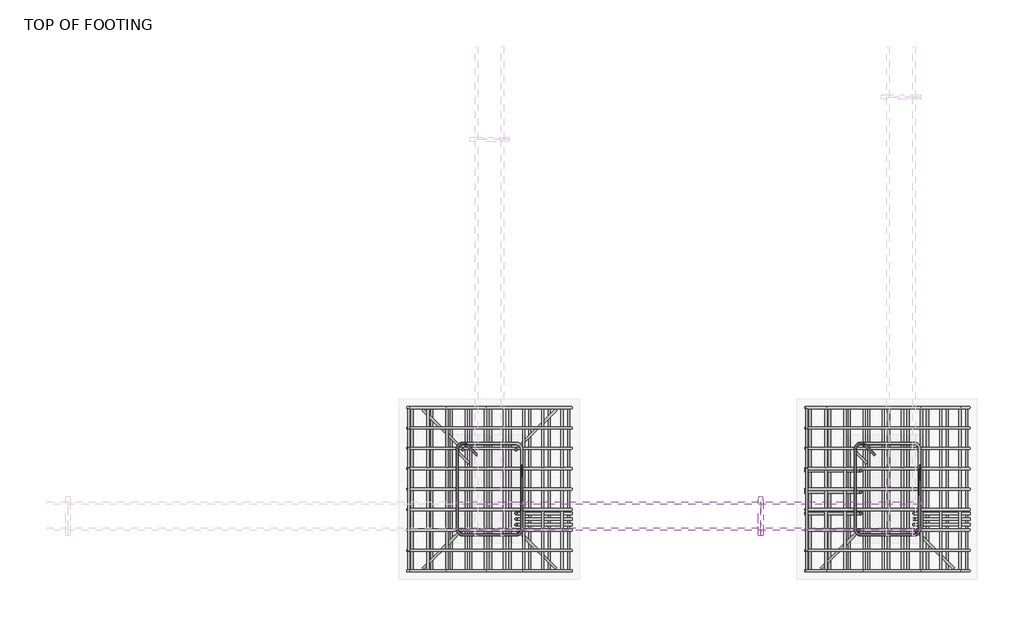
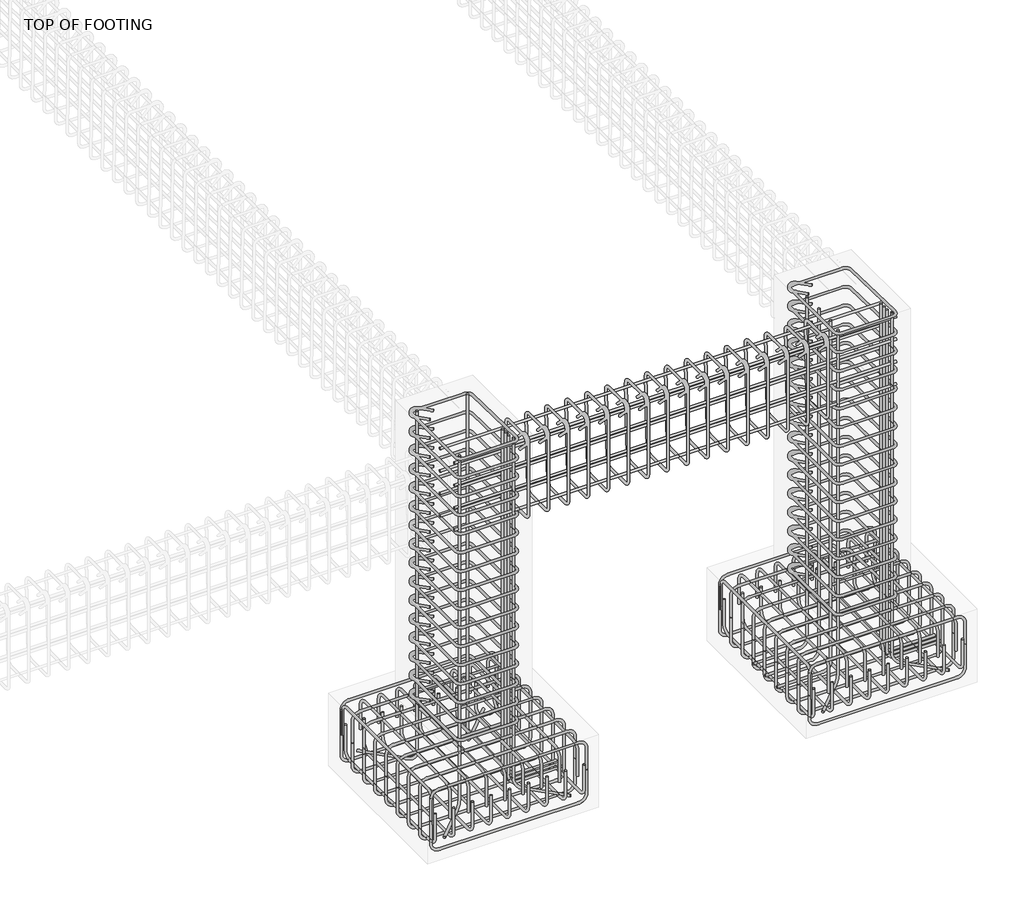
# One storey, part 4 of 9: 22 reinforcing bars.
"""IFC4 building model written with IfcOpenShell, lengths in millimetres."""

from ifc_helpers import new_model, si_unit, point, frame, origin, place, context, project, spatial, polyline, circle_curve, trimmed, segment, composite_curve, source, transform, mapped, element, save
from ifc_brep_helpers import swept_disk

model = new_model("IFC4")

# Units and contexts
model_context = context("Model", 3, world=origin())
ifc_project = project(units=[si_unit("LENGTHUNIT", "METRE", prefix="MILLI")], contexts=[model_context])

# Site, building, storey
site = spatial("IfcSite", under=ifc_project)
building = spatial("IfcBuilding", under=site)
storey = spatial("IfcBuildingStorey", under=building, Name="TOP OF FOOTING", Elevation=-1828.8)

# Reinforcing bars
placement = place(None, origin())
reinforcing_bar_shape = source(origin(), model_context, "Body", "SolidModel", [
    swept_disk(composite_curve([segment(polyline([(-1479.6174526, -598.6824927, -2052.8356656), (-1479.6174526, -598.6824927, -2200.1356656)]), True, "CONTINUOUS"), segment(trimmed(circle_curve(frame((-1525.9674526, -598.6824927, -2200.1356656), z_axis=(0.0, 1.0, 0.0), x_axis=(46.34999999999991, 0.0, 0.0)), 46.35), [point((-1479.6174526, -598.6824927, -2200.1356656))], [point((-1525.9674526, -598.6824927, -2246.4856656))], True, "CARTESIAN"), True, "CONTINUOUS"), segment(polyline([(-1525.9674526, -598.6824927, -2246.4856656), (-2340.5674526, -598.6824927, -2246.4856656)]), True, "CONTINUOUS"), segment(trimmed(circle_curve(frame((-2340.5674526, -598.6824927, -2200.1356656), z_axis=(0.0, 1.0, 0.0), x_axis=(0.0, 0.0, -46.350000000000364)), 46.35), [point((-2340.5674526, -598.6824927, -2246.4856656))], [point((-2386.9174526, -598.6824927, -2200.1356656))], True, "CARTESIAN"), True, "CONTINUOUS"), segment(polyline([(-2386.9174526, -598.6824927, -2200.1356656), (-2386.9174526, -598.6824927, -2052.8356656)]), True, "CONTINUOUS")], self_intersect=False), 6.35),
])
element("IfcReinforcingBar", 1, at=placement, inside=storey, context=model_context, shape_type="MappedRepresentation", body=[
    mapped(reinforcing_bar_shape, transform((0.0, 0.0, 0.0), x_axis=(1.0, 0.0, 0.0), y_axis=(0.0, 1.0, 0.0), z_axis=(0.0, 0.0, 1.0))),
    mapped(reinforcing_bar_shape, transform((0.0, -113.4125, 0.0), x_axis=(1.0, 0.0, 0.0), y_axis=(0.0, 1.0, 0.0), z_axis=(0.0, 0.0, 1.0))),
    mapped(reinforcing_bar_shape, transform((0.0, -226.825, 0.0), x_axis=(1.0, 0.0, 0.0), y_axis=(0.0, 1.0, 0.0), z_axis=(0.0, 0.0, 1.0))),
    mapped(reinforcing_bar_shape, transform((0.0, -340.2375, 0.0), x_axis=(1.0, 0.0, 0.0), y_axis=(0.0, 1.0, 0.0), z_axis=(0.0, 0.0, 1.0))),
    mapped(reinforcing_bar_shape, transform((0.0, -453.65, 0.0), x_axis=(1.0, 0.0, 0.0), y_axis=(0.0, 1.0, 0.0), z_axis=(0.0, 0.0, 1.0))),
    mapped(reinforcing_bar_shape, transform((0.0, -567.0625, 0.0), x_axis=(1.0, 0.0, 0.0), y_axis=(0.0, 1.0, 0.0), z_axis=(0.0, 0.0, 1.0))),
    mapped(reinforcing_bar_shape, transform((0.0, -680.475, 0.0), x_axis=(1.0, 0.0, 0.0), y_axis=(0.0, 1.0, 0.0), z_axis=(0.0, 0.0, 1.0))),
    mapped(reinforcing_bar_shape, transform((0.0, -793.8875, 0.0), x_axis=(1.0, 0.0, 0.0), y_axis=(0.0, 1.0, 0.0), z_axis=(0.0, 0.0, 1.0))),
    mapped(reinforcing_bar_shape, transform((0.0, -907.3, 0.0), x_axis=(1.0, 0.0, 0.0), y_axis=(0.0, 1.0, 0.0), z_axis=(0.0, 0.0, 1.0))),
])
reinforcing_bar_2_shape = source(origin(), model_context, "Body", "SolidModel", [
    swept_disk(composite_curve([segment(polyline([(-2386.9174526, -598.6824927, -2068.8), (-2386.9174526, -598.6824927, -1921.5)]), True, "CONTINUOUS"), segment(trimmed(circle_curve(frame((-2340.5674526, -598.6824927, -1921.5), z_axis=(0.0, 1.0, 0.0), x_axis=(-46.350000000000364, 0.0, 0.0)), 46.35), [point((-2386.9174526, -598.6824927, -1921.5))], [point((-2340.5674526, -598.6824927, -1875.15))], True, "CARTESIAN"), True, "CONTINUOUS"), segment(polyline([(-2340.5674526, -598.6824927, -1875.15), (-1525.9674526, -598.6824927, -1875.15)]), True, "CONTINUOUS"), segment(trimmed(circle_curve(frame((-1525.9674526, -598.6824927, -1921.5), z_axis=(0.0, 1.0, 0.0), x_axis=(0.0, 0.0, 46.34999999999991)), 46.35), [point((-1525.9674526, -598.6824927, -1875.15))], [point((-1479.6174526, -598.6824927, -1921.5))], True, "CARTESIAN"), True, "CONTINUOUS"), segment(polyline([(-1479.6174526, -598.6824927, -1921.5), (-1479.6174526, -598.6824927, -2068.8)]), True, "CONTINUOUS")], self_intersect=False), 6.35),
])
element("IfcReinforcingBar", 2, at=placement, inside=storey, context=model_context, shape_type="MappedRepresentation", body=[
    mapped(reinforcing_bar_2_shape, transform((0.0, 0.0, 0.0), x_axis=(1.0, 0.0, 0.0), y_axis=(0.0, 1.0, 0.0), z_axis=(0.0, 0.0, 1.0))),
    mapped(reinforcing_bar_2_shape, transform((0.0, -113.4125, 0.0), x_axis=(1.0, 0.0, 0.0), y_axis=(0.0, 1.0, 0.0), z_axis=(0.0, 0.0, 1.0))),
    mapped(reinforcing_bar_2_shape, transform((0.0, -226.825, 0.0), x_axis=(1.0, 0.0, 0.0), y_axis=(0.0, 1.0, 0.0), z_axis=(0.0, 0.0, 1.0))),
    mapped(reinforcing_bar_2_shape, transform((0.0, -340.2375, 0.0), x_axis=(1.0, 0.0, 0.0), y_axis=(0.0, 1.0, 0.0), z_axis=(0.0, 0.0, 1.0))),
    mapped(reinforcing_bar_2_shape, transform((0.0, -453.65, 0.0), x_axis=(1.0, 0.0, 0.0), y_axis=(0.0, 1.0, 0.0), z_axis=(0.0, 0.0, 1.0))),
    mapped(reinforcing_bar_2_shape, transform((0.0, -567.0625, 0.0), x_axis=(1.0, 0.0, 0.0), y_axis=(0.0, 1.0, 0.0), z_axis=(0.0, 0.0, 1.0))),
    mapped(reinforcing_bar_2_shape, transform((0.0, -680.475, 0.0), x_axis=(1.0, 0.0, 0.0), y_axis=(0.0, 1.0, 0.0), z_axis=(0.0, 0.0, 1.0))),
    mapped(reinforcing_bar_2_shape, transform((0.0, -793.8875, 0.0), x_axis=(1.0, 0.0, 0.0), y_axis=(0.0, 1.0, 0.0), z_axis=(0.0, 0.0, 1.0))),
    mapped(reinforcing_bar_2_shape, transform((0.0, -907.3, 0.0), x_axis=(1.0, 0.0, 0.0), y_axis=(0.0, 1.0, 0.0), z_axis=(0.0, 0.0, 1.0))),
])
reinforcing_bar_3_shape = source(origin(), model_context, "Body", "SolidModel", [
    swept_disk(composite_curve([segment(polyline([(-2363.2674526, -598.6824927, -2020.15), (-2363.2674526, -598.6824927, -2167.45)]), True, "CONTINUOUS"), segment(trimmed(circle_curve(frame((-2363.2674526, -645.0324927, -2167.45), z_axis=(-1.0, 0.0, 0.0), x_axis=(0.0, 46.35000000000002, 0.0)), 46.35), [point((-2363.2674526, -598.6824927, -2167.45))], [point((-2363.2674526, -645.0324927, -2213.8))], True, "CARTESIAN"), True, "CONTINUOUS"), segment(polyline([(-2363.2674526, -645.0324927, -2213.8), (-2363.2674526, -1459.6324927, -2213.8)]), True, "CONTINUOUS"), segment(trimmed(circle_curve(frame((-2363.2674526, -1459.6324927, -2167.45), z_axis=(-1.0, 0.0, 0.0), x_axis=(0.0, 0.0, -46.350000000000364)), 46.35), [point((-2363.2674526, -1459.6324927, -2213.8))], [point((-2363.2674526, -1505.9824927, -2167.45))], True, "CARTESIAN"), True, "CONTINUOUS"), segment(polyline([(-2363.2674526, -1505.9824927, -2167.45), (-2363.2674526, -1505.9824927, -2020.15)]), True, "CONTINUOUS")], self_intersect=False), 6.35),
])
element("IfcReinforcingBar", 3, at=placement, inside=storey, context=model_context, shape_type="MappedRepresentation", body=[
    mapped(reinforcing_bar_3_shape, transform((0.0, 0.0, 0.0), x_axis=(1.0, 0.0, 0.0), y_axis=(0.0, 1.0, 0.0), z_axis=(0.0, 0.0, 1.0))),
    mapped(reinforcing_bar_3_shape, transform((108.8370374, 0.0, 0.0), x_axis=(1.0, 0.0, 0.0), y_axis=(0.0, 1.0, 0.0), z_axis=(0.0, 0.0, 1.0))),
    mapped(reinforcing_bar_3_shape, transform((217.6740748, 0.0, 0.0), x_axis=(1.0, 0.0, 0.0), y_axis=(0.0, 1.0, 0.0), z_axis=(0.0, 0.0, 1.0))),
    mapped(reinforcing_bar_3_shape, transform((326.5111123, 0.0, 0.0), x_axis=(1.0, 0.0, 0.0), y_axis=(0.0, 1.0, 0.0), z_axis=(0.0, 0.0, 1.0))),
    mapped(reinforcing_bar_3_shape, transform((435.3481497, 0.0, 0.0), x_axis=(1.0, 0.0, 0.0), y_axis=(0.0, 1.0, 0.0), z_axis=(0.0, 0.0, 1.0))),
    mapped(reinforcing_bar_3_shape, transform((544.1851871, 0.0, 0.0), x_axis=(1.0, 0.0, 0.0), y_axis=(0.0, 1.0, 0.0), z_axis=(0.0, 0.0, 1.0))),
    mapped(reinforcing_bar_3_shape, transform((653.0222245, 0.0, 0.0), x_axis=(1.0, 0.0, 0.0), y_axis=(0.0, 1.0, 0.0), z_axis=(0.0, 0.0, 1.0))),
    mapped(reinforcing_bar_3_shape, transform((761.8592619, 0.0, 0.0), x_axis=(1.0, 0.0, 0.0), y_axis=(0.0, 1.0, 0.0), z_axis=(0.0, 0.0, 1.0))),
    mapped(reinforcing_bar_3_shape, transform((870.6962994, 0.0, 0.0), x_axis=(1.0, 0.0, 0.0), y_axis=(0.0, 1.0, 0.0), z_axis=(0.0, 0.0, 1.0))),
])
reinforcing_bar_4_shape = source(origin(), model_context, "Body", "SolidModel", [
    swept_disk(composite_curve([segment(polyline([(-1530.7455787, -598.6824927, -2076.9782245), (-1530.7455787, -598.6824927, -1929.6782245)]), True, "CONTINUOUS"), segment(trimmed(circle_curve(frame((-1530.7455787, -645.0324927, -1929.6782245), z_axis=(1.0, 0.0, 0.0), x_axis=(0.0, 46.35000000000002, 0.0)), 46.35), [point((-1530.7455787, -598.6824927, -1929.6782245))], [point((-1530.7455787, -645.0324927, -1883.3282245))], True, "CARTESIAN"), True, "CONTINUOUS"), segment(polyline([(-1530.7455787, -645.0324927, -1883.3282245), (-1530.7455787, -1459.6324927, -1883.3282245)]), True, "CONTINUOUS"), segment(trimmed(circle_curve(frame((-1530.7455787, -1459.6324927, -1929.6782245), z_axis=(1.0, 0.0, 0.0), x_axis=(0.0, 0.0, 46.34999999999991)), 46.35), [point((-1530.7455787, -1459.6324927, -1883.3282245))], [point((-1530.7455787, -1505.9824927, -1929.6782245))], True, "CARTESIAN"), True, "CONTINUOUS"), segment(polyline([(-1530.7455787, -1505.9824927, -1929.6782245), (-1530.7455787, -1505.9824927, -2076.9782245)]), True, "CONTINUOUS")], self_intersect=False), 6.35),
])
element("IfcReinforcingBar", 4, at=placement, inside=storey, context=model_context, shape_type="MappedRepresentation", body=[
    mapped(reinforcing_bar_4_shape, transform((0.0, 0.0, 0.0), x_axis=(1.0, 0.0, 0.0), y_axis=(0.0, 1.0, 0.0), z_axis=(0.0, 0.0, 1.0))),
    mapped(reinforcing_bar_4_shape, transform((-106.3275638, 0.0, 0.0), x_axis=(1.0, 0.0, 0.0), y_axis=(0.0, 1.0, 0.0), z_axis=(0.0, 0.0, 1.0))),
    mapped(reinforcing_bar_4_shape, transform((-212.6551275, 0.0, 0.0), x_axis=(1.0, 0.0, 0.0), y_axis=(0.0, 1.0, 0.0), z_axis=(0.0, 0.0, 1.0))),
    mapped(reinforcing_bar_4_shape, transform((-318.9826913, 0.0, 0.0), x_axis=(1.0, 0.0, 0.0), y_axis=(0.0, 1.0, 0.0), z_axis=(0.0, 0.0, 1.0))),
    mapped(reinforcing_bar_4_shape, transform((-425.310255, 0.0, 0.0), x_axis=(1.0, 0.0, 0.0), y_axis=(0.0, 1.0, 0.0), z_axis=(0.0, 0.0, 1.0))),
    mapped(reinforcing_bar_4_shape, transform((-531.6378188, 0.0, 0.0), x_axis=(1.0, 0.0, 0.0), y_axis=(0.0, 1.0, 0.0), z_axis=(0.0, 0.0, 1.0))),
    mapped(reinforcing_bar_4_shape, transform((-637.9653825, 0.0, 0.0), x_axis=(1.0, 0.0, 0.0), y_axis=(0.0, 1.0, 0.0), z_axis=(0.0, 0.0, 1.0))),
    mapped(reinforcing_bar_4_shape, transform((-744.2929463, 0.0, 0.0), x_axis=(1.0, 0.0, 0.0), y_axis=(0.0, 1.0, 0.0), z_axis=(0.0, 0.0, 1.0))),
    mapped(reinforcing_bar_4_shape, transform((-850.62051, 0.0, 0.0), x_axis=(1.0, 0.0, 0.0), y_axis=(0.0, 1.0, 0.0), z_axis=(0.0, 0.0, 1.0))),
])
reinforcing_bar_5_shape = source(origin(), model_context, "Body", "SolidModel", [
    swept_disk(composite_curve([segment(polyline([(730.3825474, -598.6824927, -2052.8356656), (730.3825474, -598.6824927, -2200.1356656)]), True, "CONTINUOUS"), segment(trimmed(circle_curve(frame((684.0325474, -598.6824927, -2200.1356656), z_axis=(0.0, 1.0, 0.0), x_axis=(46.35000000000002, 0.0, 0.0)), 46.35), [point((730.3825474, -598.6824927, -2200.1356656))], [point((684.0325474, -598.6824927, -2246.4856656))], True, "CARTESIAN"), True, "CONTINUOUS"), segment(polyline([(684.0325474, -598.6824927, -2246.4856656), (-130.5674526, -598.6824927, -2246.4856656)]), True, "CONTINUOUS"), segment(trimmed(circle_curve(frame((-130.5674526, -598.6824927, -2200.1356656), z_axis=(0.0, 1.0, 0.0), x_axis=(0.0, 0.0, -46.350000000000364)), 46.35), [point((-130.5674526, -598.6824927, -2246.4856656))], [point((-176.9174526, -598.6824927, -2200.1356656))], True, "CARTESIAN"), True, "CONTINUOUS"), segment(polyline([(-176.9174526, -598.6824927, -2200.1356656), (-176.9174526, -598.6824927, -2052.8356656)]), True, "CONTINUOUS")], self_intersect=False), 6.35),
])
element("IfcReinforcingBar", 5, at=placement, inside=storey, context=model_context, shape_type="MappedRepresentation", body=[
    mapped(reinforcing_bar_5_shape, transform((0.0, 0.0, 0.0), x_axis=(1.0, 0.0, 0.0), y_axis=(0.0, 1.0, 0.0), z_axis=(0.0, 0.0, 1.0))),
    mapped(reinforcing_bar_5_shape, transform((0.0, -113.4125, 0.0), x_axis=(1.0, 0.0, 0.0), y_axis=(0.0, 1.0, 0.0), z_axis=(0.0, 0.0, 1.0))),
    mapped(reinforcing_bar_5_shape, transform((0.0, -226.825, 0.0), x_axis=(1.0, 0.0, 0.0), y_axis=(0.0, 1.0, 0.0), z_axis=(0.0, 0.0, 1.0))),
    mapped(reinforcing_bar_5_shape, transform((0.0, -340.2375, 0.0), x_axis=(1.0, 0.0, 0.0), y_axis=(0.0, 1.0, 0.0), z_axis=(0.0, 0.0, 1.0))),
    mapped(reinforcing_bar_5_shape, transform((0.0, -453.65, 0.0), x_axis=(1.0, 0.0, 0.0), y_axis=(0.0, 1.0, 0.0), z_axis=(0.0, 0.0, 1.0))),
    mapped(reinforcing_bar_5_shape, transform((0.0, -567.0625, 0.0), x_axis=(1.0, 0.0, 0.0), y_axis=(0.0, 1.0, 0.0), z_axis=(0.0, 0.0, 1.0))),
    mapped(reinforcing_bar_5_shape, transform((0.0, -680.475, 0.0), x_axis=(1.0, 0.0, 0.0), y_axis=(0.0, 1.0, 0.0), z_axis=(0.0, 0.0, 1.0))),
    mapped(reinforcing_bar_5_shape, transform((0.0, -793.8875, 0.0), x_axis=(1.0, 0.0, 0.0), y_axis=(0.0, 1.0, 0.0), z_axis=(0.0, 0.0, 1.0))),
    mapped(reinforcing_bar_5_shape, transform((0.0, -907.3, 0.0), x_axis=(1.0, 0.0, 0.0), y_axis=(0.0, 1.0, 0.0), z_axis=(0.0, 0.0, 1.0))),
])
reinforcing_bar_6_shape = source(origin(), model_context, "Body", "SolidModel", [
    swept_disk(composite_curve([segment(polyline([(-176.9174526, -598.6824927, -2068.8), (-176.9174526, -598.6824927, -1921.5)]), True, "CONTINUOUS"), segment(trimmed(circle_curve(frame((-130.5674526, -598.6824927, -1921.5), z_axis=(0.0, 1.0, 0.0), x_axis=(-46.349999999999994, 0.0, 0.0)), 46.35), [point((-176.9174526, -598.6824927, -1921.5))], [point((-130.5674526, -598.6824927, -1875.15))], True, "CARTESIAN"), True, "CONTINUOUS"), segment(polyline([(-130.5674526, -598.6824927, -1875.15), (684.0325474, -598.6824927, -1875.15)]), True, "CONTINUOUS"), segment(trimmed(circle_curve(frame((684.0325474, -598.6824927, -1921.5), z_axis=(0.0, 1.0, 0.0), x_axis=(0.0, 0.0, 46.34999999999991)), 46.35), [point((684.0325474, -598.6824927, -1875.15))], [point((730.3825474, -598.6824927, -1921.5))], True, "CARTESIAN"), True, "CONTINUOUS"), segment(polyline([(730.3825474, -598.6824927, -1921.5), (730.3825474, -598.6824927, -2068.8)]), True, "CONTINUOUS")], self_intersect=False), 6.35),
])
element("IfcReinforcingBar", 6, at=placement, inside=storey, context=model_context, shape_type="MappedRepresentation", body=[
    mapped(reinforcing_bar_6_shape, transform((0.0, 0.0, 0.0), x_axis=(1.0, 0.0, 0.0), y_axis=(0.0, 1.0, 0.0), z_axis=(0.0, 0.0, 1.0))),
    mapped(reinforcing_bar_6_shape, transform((0.0, -113.4125, 0.0), x_axis=(1.0, 0.0, 0.0), y_axis=(0.0, 1.0, 0.0), z_axis=(0.0, 0.0, 1.0))),
    mapped(reinforcing_bar_6_shape, transform((0.0, -226.825, 0.0), x_axis=(1.0, 0.0, 0.0), y_axis=(0.0, 1.0, 0.0), z_axis=(0.0, 0.0, 1.0))),
    mapped(reinforcing_bar_6_shape, transform((0.0, -340.2375, 0.0), x_axis=(1.0, 0.0, 0.0), y_axis=(0.0, 1.0, 0.0), z_axis=(0.0, 0.0, 1.0))),
    mapped(reinforcing_bar_6_shape, transform((0.0, -453.65, 0.0), x_axis=(1.0, 0.0, 0.0), y_axis=(0.0, 1.0, 0.0), z_axis=(0.0, 0.0, 1.0))),
    mapped(reinforcing_bar_6_shape, transform((0.0, -567.0625, 0.0), x_axis=(1.0, 0.0, 0.0), y_axis=(0.0, 1.0, 0.0), z_axis=(0.0, 0.0, 1.0))),
    mapped(reinforcing_bar_6_shape, transform((0.0, -680.475, 0.0), x_axis=(1.0, 0.0, 0.0), y_axis=(0.0, 1.0, 0.0), z_axis=(0.0, 0.0, 1.0))),
    mapped(reinforcing_bar_6_shape, transform((0.0, -793.8875, 0.0), x_axis=(1.0, 0.0, 0.0), y_axis=(0.0, 1.0, 0.0), z_axis=(0.0, 0.0, 1.0))),
    mapped(reinforcing_bar_6_shape, transform((0.0, -907.3, 0.0), x_axis=(1.0, 0.0, 0.0), y_axis=(0.0, 1.0, 0.0), z_axis=(0.0, 0.0, 1.0))),
])
reinforcing_bar_7_shape = source(origin(), model_context, "Body", "SolidModel", [
    swept_disk(composite_curve([segment(polyline([(-153.2674526, -598.6824927, -2020.15), (-153.2674526, -598.6824927, -2167.45)]), True, "CONTINUOUS"), segment(trimmed(circle_curve(frame((-153.2674526, -645.0324927, -2167.45), z_axis=(-1.0, 0.0, 0.0), x_axis=(0.0, 46.35000000000002, 0.0)), 46.35), [point((-153.2674526, -598.6824927, -2167.45))], [point((-153.2674526, -645.0324927, -2213.8))], True, "CARTESIAN"), True, "CONTINUOUS"), segment(polyline([(-153.2674526, -645.0324927, -2213.8), (-153.2674526, -1459.6324927, -2213.8)]), True, "CONTINUOUS"), segment(trimmed(circle_curve(frame((-153.2674526, -1459.6324927, -2167.45), z_axis=(-1.0, 0.0, 0.0), x_axis=(0.0, 0.0, -46.350000000000364)), 46.35), [point((-153.2674526, -1459.6324927, -2213.8))], [point((-153.2674526, -1505.9824927, -2167.45))], True, "CARTESIAN"), True, "CONTINUOUS"), segment(polyline([(-153.2674526, -1505.9824927, -2167.45), (-153.2674526, -1505.9824927, -2020.15)]), True, "CONTINUOUS")], self_intersect=False), 6.35),
])
element("IfcReinforcingBar", 7, at=placement, inside=storey, context=model_context, shape_type="MappedRepresentation", body=[
    mapped(reinforcing_bar_7_shape, transform((0.0, 0.0, 0.0), x_axis=(1.0, 0.0, 0.0), y_axis=(0.0, 1.0, 0.0), z_axis=(0.0, 0.0, 1.0))),
    mapped(reinforcing_bar_7_shape, transform((108.8370374, 0.0, 0.0), x_axis=(1.0, 0.0, 0.0), y_axis=(0.0, 1.0, 0.0), z_axis=(0.0, 0.0, 1.0))),
    mapped(reinforcing_bar_7_shape, transform((217.6740748, 0.0, 0.0), x_axis=(1.0, 0.0, 0.0), y_axis=(0.0, 1.0, 0.0), z_axis=(0.0, 0.0, 1.0))),
    mapped(reinforcing_bar_7_shape, transform((326.5111123, 0.0, 0.0), x_axis=(1.0, 0.0, 0.0), y_axis=(0.0, 1.0, 0.0), z_axis=(0.0, 0.0, 1.0))),
    mapped(reinforcing_bar_7_shape, transform((435.3481497, 0.0, 0.0), x_axis=(1.0, 0.0, 0.0), y_axis=(0.0, 1.0, 0.0), z_axis=(0.0, 0.0, 1.0))),
    mapped(reinforcing_bar_7_shape, transform((544.1851871, 0.0, 0.0), x_axis=(1.0, 0.0, 0.0), y_axis=(0.0, 1.0, 0.0), z_axis=(0.0, 0.0, 1.0))),
    mapped(reinforcing_bar_7_shape, transform((653.0222245, 0.0, 0.0), x_axis=(1.0, 0.0, 0.0), y_axis=(0.0, 1.0, 0.0), z_axis=(0.0, 0.0, 1.0))),
    mapped(reinforcing_bar_7_shape, transform((761.8592619, 0.0, 0.0), x_axis=(1.0, 0.0, 0.0), y_axis=(0.0, 1.0, 0.0), z_axis=(0.0, 0.0, 1.0))),
    mapped(reinforcing_bar_7_shape, transform((870.6962994, 0.0, 0.0), x_axis=(1.0, 0.0, 0.0), y_axis=(0.0, 1.0, 0.0), z_axis=(0.0, 0.0, 1.0))),
])
reinforcing_bar_8_shape = source(origin(), model_context, "Body", "SolidModel", [
    swept_disk(composite_curve([segment(polyline([(679.2544213, -598.6824927, -2076.9782245), (679.2544213, -598.6824927, -1929.6782245)]), True, "CONTINUOUS"), segment(trimmed(circle_curve(frame((679.2544213, -645.0324927, -1929.6782245), z_axis=(1.0, 0.0, 0.0), x_axis=(0.0, 46.35000000000002, 0.0)), 46.35), [point((679.2544213, -598.6824927, -1929.6782245))], [point((679.2544213, -645.0324927, -1883.3282245))], True, "CARTESIAN"), True, "CONTINUOUS"), segment(polyline([(679.2544213, -645.0324927, -1883.3282245), (679.2544213, -1459.6324927, -1883.3282245)]), True, "CONTINUOUS"), segment(trimmed(circle_curve(frame((679.2544213, -1459.6324927, -1929.6782245), z_axis=(1.0, 0.0, 0.0), x_axis=(0.0, 0.0, 46.34999999999991)), 46.35), [point((679.2544213, -1459.6324927, -1883.3282245))], [point((679.2544213, -1505.9824927, -1929.6782245))], True, "CARTESIAN"), True, "CONTINUOUS"), segment(polyline([(679.2544213, -1505.9824927, -1929.6782245), (679.2544213, -1505.9824927, -2076.9782245)]), True, "CONTINUOUS")], self_intersect=False), 6.35),
])
element("IfcReinforcingBar", 8, at=placement, inside=storey, context=model_context, shape_type="MappedRepresentation", body=[
    mapped(reinforcing_bar_8_shape, transform((0.0, 0.0, 0.0), x_axis=(1.0, 0.0, 0.0), y_axis=(0.0, 1.0, 0.0), z_axis=(0.0, 0.0, 1.0))),
    mapped(reinforcing_bar_8_shape, transform((-106.3275638, 0.0, 0.0), x_axis=(1.0, 0.0, 0.0), y_axis=(0.0, 1.0, 0.0), z_axis=(0.0, 0.0, 1.0))),
    mapped(reinforcing_bar_8_shape, transform((-212.6551275, 0.0, 0.0), x_axis=(1.0, 0.0, 0.0), y_axis=(0.0, 1.0, 0.0), z_axis=(0.0, 0.0, 1.0))),
    mapped(reinforcing_bar_8_shape, transform((-318.9826913, 0.0, 0.0), x_axis=(1.0, 0.0, 0.0), y_axis=(0.0, 1.0, 0.0), z_axis=(0.0, 0.0, 1.0))),
    mapped(reinforcing_bar_8_shape, transform((-425.310255, 0.0, 0.0), x_axis=(1.0, 0.0, 0.0), y_axis=(0.0, 1.0, 0.0), z_axis=(0.0, 0.0, 1.0))),
    mapped(reinforcing_bar_8_shape, transform((-531.6378188, 0.0, 0.0), x_axis=(1.0, 0.0, 0.0), y_axis=(0.0, 1.0, 0.0), z_axis=(0.0, 0.0, 1.0))),
    mapped(reinforcing_bar_8_shape, transform((-637.9653825, 0.0, 0.0), x_axis=(1.0, 0.0, 0.0), y_axis=(0.0, 1.0, 0.0), z_axis=(0.0, 0.0, 1.0))),
    mapped(reinforcing_bar_8_shape, transform((-744.2929463, 0.0, 0.0), x_axis=(1.0, 0.0, 0.0), y_axis=(0.0, 1.0, 0.0), z_axis=(0.0, 0.0, 1.0))),
    mapped(reinforcing_bar_8_shape, transform((-850.62051, 0.0, 0.0), x_axis=(1.0, 0.0, 0.0), y_axis=(0.0, 1.0, 0.0), z_axis=(0.0, 0.0, 1.0))),
])
reinforcing_bar_9_shape = source(origin(), model_context, "Body", "SolidModel", [
    swept_disk(composite_curve([segment(polyline([(-2002.6560921, -863.6082581, -1782.45), (-2058.399655, -807.8646951, -1782.45)]), True, "CONTINUOUS"), segment(trimmed(circle_curve(frame((-2080.5674526, -830.0324927, -1782.45), z_axis=(0.0, 0.0, 1.0), x_axis=(22.16779759999963, 22.167797600000085, 0.0)), 31.35), [point((-2058.399655, -807.8646951, -1782.45))], [point((-2111.9174526, -830.0324927, -1782.45))], True, "CARTESIAN"), True, "CONTINUOUS"), segment(polyline([(-2111.9174526, -830.0324927, -1782.45), (-2111.9174526, -1274.6324927, -1782.45)]), True, "CONTINUOUS"), segment(trimmed(circle_curve(frame((-2080.5674526, -1274.6324927, -1782.45), z_axis=(0.0, 0.0, 1.0), x_axis=(-31.350000000000364, 0.0, 0.0)), 31.35), [point((-2111.9174526, -1274.6324927, -1782.45))], [point((-2080.5674526, -1305.9824927, -1782.45))], True, "CARTESIAN"), True, "CONTINUOUS"), segment(polyline([(-2080.5674526, -1305.9824927, -1782.45), (-1785.9674526, -1305.9824927, -1782.45)]), True, "CONTINUOUS"), segment(trimmed(circle_curve(frame((-1785.9674526, -1274.642312, -1783.2345856), z_axis=(0.0, 0.025026655153786315, 0.9996867842138424), x_axis=(0.0, -31.34018070000002, 0.7845855999999003)), 31.35), [point((-1785.9674526, -1305.9824927, -1782.45))], [point((-1754.6174526, -1274.642312, -1783.2345856))], True, "CARTESIAN"), True, "CONTINUOUS"), segment(polyline([(-1754.6174526, -1274.642312, -1783.2345856), (-1754.6174526, -830.0226734, -1794.3654144)]), True, "CONTINUOUS"), segment(trimmed(circle_curve(frame((-1785.9674526, -830.0226734, -1794.3654144), z_axis=(0.0, 0.025026655153786315, 0.9996867842138424), x_axis=(31.34999999999991, 0.0, 0.0)), 31.35), [point((-1754.6174526, -830.0226734, -1794.3654144))], [point((-1785.9674526, -798.6824927, -1795.15))], True, "CARTESIAN"), True, "CONTINUOUS"), segment(polyline([(-1785.9674526, -798.6824927, -1795.15), (-2080.5674526, -798.6824927, -1795.15)]), True, "CONTINUOUS"), segment(trimmed(circle_curve(frame((-2080.5674526, -830.0324927, -1795.15), z_axis=(0.0, 0.0, 1.0), x_axis=(0.0, 31.350000000000023, 0.0)), 31.35), [point((-2080.5674526, -798.6824927, -1795.15))], [point((-2102.7352502, -852.2002903, -1795.15))], True, "CARTESIAN"), True, "CONTINUOUS"), segment(polyline([(-2102.7352502, -852.2002903, -1795.15), (-2046.9916873, -907.9438533, -1795.15)]), True, "CONTINUOUS")], self_intersect=False), 6.35),
])
element("IfcReinforcingBar", 9, at=placement, inside=storey, context=model_context, shape_type="MappedRepresentation", body=[
    mapped(reinforcing_bar_9_shape, transform((0.0, 0.0, 0.0), x_axis=(1.0, 0.0, 0.0), y_axis=(0.0, 1.0, 0.0), z_axis=(0.0, 0.0, 1.0))),
    mapped(reinforcing_bar_9_shape, transform((0.0, 0.0, 115.74), x_axis=(1.0, 0.0, 0.0), y_axis=(0.0, 1.0, 0.0), z_axis=(0.0, 0.0, 1.0))),
    mapped(reinforcing_bar_9_shape, transform((0.0, 0.0, 231.48), x_axis=(1.0, 0.0, 0.0), y_axis=(0.0, 1.0, 0.0), z_axis=(0.0, 0.0, 1.0))),
    mapped(reinforcing_bar_9_shape, transform((0.0, 0.0, 347.22), x_axis=(1.0, 0.0, 0.0), y_axis=(0.0, 1.0, 0.0), z_axis=(0.0, 0.0, 1.0))),
    mapped(reinforcing_bar_9_shape, transform((0.0, 0.0, 462.96), x_axis=(1.0, 0.0, 0.0), y_axis=(0.0, 1.0, 0.0), z_axis=(0.0, 0.0, 1.0))),
    mapped(reinforcing_bar_9_shape, transform((0.0, 0.0, 578.7), x_axis=(1.0, 0.0, 0.0), y_axis=(0.0, 1.0, 0.0), z_axis=(0.0, 0.0, 1.0))),
    mapped(reinforcing_bar_9_shape, transform((0.0, 0.0, 694.44), x_axis=(1.0, 0.0, 0.0), y_axis=(0.0, 1.0, 0.0), z_axis=(0.0, 0.0, 1.0))),
    mapped(reinforcing_bar_9_shape, transform((0.0, 0.0, 810.18), x_axis=(1.0, 0.0, 0.0), y_axis=(0.0, 1.0, 0.0), z_axis=(0.0, 0.0, 1.0))),
    mapped(reinforcing_bar_9_shape, transform((0.0, 0.0, 925.92), x_axis=(1.0, 0.0, 0.0), y_axis=(0.0, 1.0, 0.0), z_axis=(0.0, 0.0, 1.0))),
    mapped(reinforcing_bar_9_shape, transform((0.0, 0.0, 1041.66), x_axis=(1.0, 0.0, 0.0), y_axis=(0.0, 1.0, 0.0), z_axis=(0.0, 0.0, 1.0))),
    mapped(reinforcing_bar_9_shape, transform((0.0, 0.0, 1157.4), x_axis=(1.0, 0.0, 0.0), y_axis=(0.0, 1.0, 0.0), z_axis=(0.0, 0.0, 1.0))),
    mapped(reinforcing_bar_9_shape, transform((0.0, 0.0, 1273.14), x_axis=(1.0, 0.0, 0.0), y_axis=(0.0, 1.0, 0.0), z_axis=(0.0, 0.0, 1.0))),
    mapped(reinforcing_bar_9_shape, transform((0.0, 0.0, 1388.88), x_axis=(1.0, 0.0, 0.0), y_axis=(0.0, 1.0, 0.0), z_axis=(0.0, 0.0, 1.0))),
    mapped(reinforcing_bar_9_shape, transform((0.0, 0.0, 1504.62), x_axis=(1.0, 0.0, 0.0), y_axis=(0.0, 1.0, 0.0), z_axis=(0.0, 0.0, 1.0))),
    mapped(reinforcing_bar_9_shape, transform((0.0, 0.0, 1620.36), x_axis=(1.0, 0.0, 0.0), y_axis=(0.0, 1.0, 0.0), z_axis=(0.0, 0.0, 1.0))),
    mapped(reinforcing_bar_9_shape, transform((0.0, 0.0, 1736.1), x_axis=(1.0, 0.0, 0.0), y_axis=(0.0, 1.0, 0.0), z_axis=(0.0, 0.0, 1.0))),
])
element("IfcReinforcingBar", 10, at=placement, inside=storey, context=model_context, shape_type="SolidModel", body=[
    swept_disk(composite_curve([segment(polyline([(-2080.5674526, -832.8986176, -40.0), (-2080.5674526, -832.8986176, -2148.1729582)]), True, "CONTINUOUS"), segment(trimmed(circle_curve(frame((-2113.3418519, -800.1242183, -2148.1729582), z_axis=(0.7071067811865507, 0.7071067811865444, 0.0), x_axis=(32.77439930000037, -32.774399299999914, 0.0)), 46.35), [point((-2080.5674526, -832.8986176, -2148.1729582))], [point((-2113.3418519, -800.1242183, -2194.5229582))], True, "CARTESIAN"), True, "CONTINUOUS"), segment(polyline([(-2113.3418519, -800.1242183, -2194.5229582), (-2301.8537093, -611.6123609, -2194.5229582)]), True, "CONTINUOUS")], self_intersect=False), 6.35),
])
element("IfcReinforcingBar", 11, at=placement, inside=storey, context=model_context, shape_type="SolidModel", body=[
    swept_disk(composite_curve([segment(polyline([(-2090.5132324, -1281.7121476, -40.0), (-2090.5132324, -1281.7121476, -2148.1729582)]), True, "CONTINUOUS"), segment(trimmed(circle_curve(frame((-2123.2876317, -1314.4865469, -2148.1729582), z_axis=(-0.707106781186547, 0.707106781186548, 0.0), x_axis=(32.774399299999914, 32.774399299999914, 0.0)), 46.35), [point((-2090.5132324, -1281.7121476, -2148.1729582))], [point((-2123.2876317, -1314.4865469, -2194.5229582))], True, "CARTESIAN"), True, "CONTINUOUS"), segment(polyline([(-2123.2876317, -1314.4865469, -2194.5229582), (-2301.8537093, -1493.0526245, -2194.5229582)]), True, "CONTINUOUS")], self_intersect=False), 6.35),
])
element("IfcReinforcingBar", 12, at=placement, inside=storey, context=model_context, shape_type="SolidModel", body=[
    swept_disk(composite_curve([segment(polyline([(-1785.9674526, -832.8986176, -40.0), (-1785.9674526, -832.8986176, -2148.1729582)]), True, "CONTINUOUS"), segment(trimmed(circle_curve(frame((-1753.1930533, -800.1242183, -2148.1729582), z_axis=(0.7071067811865507, -0.7071067811865444, 0.0), x_axis=(-32.774399299999914, -32.774399299999914, 0.0)), 46.35), [point((-1785.9674526, -832.8986176, -2148.1729582))], [point((-1753.1930533, -800.1242183, -2194.5229582))], True, "CARTESIAN"), True, "CONTINUOUS"), segment(polyline([(-1753.1930533, -800.1242183, -2194.5229582), (-1564.6811959, -611.6123609, -2194.5229582)]), True, "CONTINUOUS")], self_intersect=False), 6.35),
])
element("IfcReinforcingBar", 13, at=placement, inside=storey, context=model_context, shape_type="SolidModel", body=[
    swept_disk(composite_curve([segment(polyline([(-1776.0216728, -1281.7121476, -40.0), (-1776.0216728, -1281.7121476, -2148.1729582)]), True, "CONTINUOUS"), segment(trimmed(circle_curve(frame((-1743.2472735, -1314.4865469, -2148.1729582), z_axis=(-0.707106781186547, -0.707106781186548, 0.0), x_axis=(-32.77439930000014, 32.774399299999914, 0.0)), 46.35), [point((-1776.0216728, -1281.7121476, -2148.1729582))], [point((-1743.2472735, -1314.4865469, -2194.5229582))], True, "CARTESIAN"), True, "CONTINUOUS"), segment(polyline([(-1743.2472735, -1314.4865469, -2194.5229582), (-1564.6811959, -1493.0526245, -2194.5229582)]), True, "CONTINUOUS")], self_intersect=False), 6.35),
])
reinforcing_bar_10_shape = source(origin(), model_context, "Body", "SolidModel", [
    swept_disk(composite_curve([segment(polyline([(-1785.9674526, -1187.8357134, -40.0), (-1785.9674526, -1187.8357134, -2148.1729582)]), True, "CONTINUOUS"), segment(trimmed(circle_curve(frame((-1739.6174526, -1187.8357134, -2148.1729582), z_axis=(0.0, -1.0, 0.0), x_axis=(-46.34999999999991, 0.0, 0.0)), 46.35), [point((-1785.9674526, -1187.8357134, -2148.1729582))], [point((-1739.6174526, -1187.8357134, -2194.5229582))], True, "CARTESIAN"), True, "CONTINUOUS"), segment(polyline([(-1739.6174526, -1187.8357134, -2194.5229582), (-1473.0214272, -1187.8357134, -2194.5229582)]), True, "CONTINUOUS")], self_intersect=False), 6.35),
])
element("IfcReinforcingBar", 14, at=placement, inside=storey, context=model_context, shape_type="MappedRepresentation", body=[
    mapped(reinforcing_bar_10_shape, transform((0.0, 0.0, 0.0), x_axis=(1.0, 0.0, 0.0), y_axis=(0.0, 1.0, 0.0), z_axis=(0.0, 0.0, 1.0))),
    mapped(reinforcing_bar_10_shape, transform((0.0, -30.8635533, 0.0), x_axis=(1.0, 0.0, 0.0), y_axis=(0.0, 1.0, 0.0), z_axis=(0.0, 0.0, 1.0))),
    mapped(reinforcing_bar_10_shape, transform((0.0, -61.7271066, 0.0), x_axis=(1.0, 0.0, 0.0), y_axis=(0.0, 1.0, 0.0), z_axis=(0.0, 0.0, 1.0))),
])
reinforcing_bar_11_shape = source(origin(), model_context, "Body", "SolidModel", [
    swept_disk(composite_curve([segment(polyline([(129.4325474, -1187.8357134, -40.0), (129.4325474, -1187.8357134, -2148.1729582)]), True, "CONTINUOUS"), segment(trimmed(circle_curve(frame((83.0825474, -1187.8357134, -2148.1729582), z_axis=(0.0, 1.0, 0.0), x_axis=(46.35000000000001, 0.0, 0.0)), 46.35), [point((129.4325474, -1187.8357134, -2148.1729582))], [point((83.0825474, -1187.8357134, -2194.5229582))], True, "CARTESIAN"), True, "CONTINUOUS"), segment(polyline([(83.0825474, -1187.8357134, -2194.5229582), (-183.513478, -1187.8357134, -2194.5229582)]), True, "CONTINUOUS")], self_intersect=False), 6.35),
])
element("IfcReinforcingBar", 15, at=placement, inside=storey, context=model_context, shape_type="MappedRepresentation", body=[
    mapped(reinforcing_bar_11_shape, transform((0.0, 0.0, 0.0), x_axis=(1.0, 0.0, 0.0), y_axis=(0.0, 1.0, 0.0), z_axis=(0.0, 0.0, 1.0))),
    mapped(reinforcing_bar_11_shape, transform((0.0, 119.1364467, 0.0), x_axis=(1.0, 0.0, 0.0), y_axis=(0.0, 1.0, 0.0), z_axis=(0.0, 0.0, 1.0))),
    mapped(reinforcing_bar_11_shape, transform((0.0, 238.2728934, 0.0), x_axis=(1.0, 0.0, 0.0), y_axis=(0.0, 1.0, 0.0), z_axis=(0.0, 0.0, 1.0))),
])
reinforcing_bar_12_shape = source(origin(), model_context, "Body", "SolidModel", [
    swept_disk(composite_curve([segment(polyline([(207.3439079, -863.6082581, -1782.45), (151.600345, -807.8646951, -1782.45)]), True, "CONTINUOUS"), segment(trimmed(circle_curve(frame((129.4325474, -830.0324927, -1782.45), z_axis=(0.0, 0.0, 1.0), x_axis=(22.1677976, 22.167797600000085, 0.0)), 31.35), [point((151.600345, -807.8646951, -1782.45))], [point((98.0825474, -830.0324927, -1782.45))], True, "CARTESIAN"), True, "CONTINUOUS"), segment(polyline([(98.0825474, -830.0324927, -1782.45), (98.0825474, -1274.6324927, -1782.45)]), True, "CONTINUOUS"), segment(trimmed(circle_curve(frame((129.4325474, -1274.6324927, -1782.45), z_axis=(0.0, 0.0, 1.0), x_axis=(-31.35000000000001, 0.0, 0.0)), 31.35), [point((98.0825474, -1274.6324927, -1782.45))], [point((129.4325474, -1305.9824927, -1782.45))], True, "CARTESIAN"), True, "CONTINUOUS"), segment(polyline([(129.4325474, -1305.9824927, -1782.45), (424.0325474, -1305.9824927, -1782.45)]), True, "CONTINUOUS"), segment(trimmed(circle_curve(frame((424.0325474, -1274.642312, -1783.2345856), z_axis=(0.0, 0.025026655153786315, 0.9996867842138424), x_axis=(0.0, -31.34018070000002, 0.7845855999999003)), 31.35), [point((424.0325474, -1305.9824927, -1782.45))], [point((455.3825474, -1274.642312, -1783.2345856))], True, "CARTESIAN"), True, "CONTINUOUS"), segment(polyline([(455.3825474, -1274.642312, -1783.2345856), (455.3825474, -830.0226734, -1794.3654144)]), True, "CONTINUOUS"), segment(trimmed(circle_curve(frame((424.0325474, -830.0226734, -1794.3654144), z_axis=(0.0, 0.025026655153786315, 0.9996867842138424), x_axis=(31.350000000000023, 0.0, 0.0)), 31.35), [point((455.3825474, -830.0226734, -1794.3654144))], [point((424.0325474, -798.6824927, -1795.15))], True, "CARTESIAN"), True, "CONTINUOUS"), segment(polyline([(424.0325474, -798.6824927, -1795.15), (129.4325474, -798.6824927, -1795.15)]), True, "CONTINUOUS"), segment(trimmed(circle_curve(frame((129.4325474, -830.0324927, -1795.15), z_axis=(0.0, 0.0, 1.0), x_axis=(0.0, 31.350000000000023, 0.0)), 31.35), [point((129.4325474, -798.6824927, -1795.15))], [point((107.2647498, -852.2002903, -1795.15))], True, "CARTESIAN"), True, "CONTINUOUS"), segment(polyline([(107.2647498, -852.2002903, -1795.15), (163.0083127, -907.9438533, -1795.15)]), True, "CONTINUOUS")], self_intersect=False), 6.35),
])
element("IfcReinforcingBar", 16, at=placement, inside=storey, context=model_context, shape_type="MappedRepresentation", body=[
    mapped(reinforcing_bar_12_shape, transform((0.0, 0.0, 0.0), x_axis=(1.0, 0.0, 0.0), y_axis=(0.0, 1.0, 0.0), z_axis=(0.0, 0.0, 1.0))),
    mapped(reinforcing_bar_12_shape, transform((0.0, 0.0, 115.74), x_axis=(1.0, 0.0, 0.0), y_axis=(0.0, 1.0, 0.0), z_axis=(0.0, 0.0, 1.0))),
    mapped(reinforcing_bar_12_shape, transform((0.0, 0.0, 231.48), x_axis=(1.0, 0.0, 0.0), y_axis=(0.0, 1.0, 0.0), z_axis=(0.0, 0.0, 1.0))),
    mapped(reinforcing_bar_12_shape, transform((0.0, 0.0, 347.22), x_axis=(1.0, 0.0, 0.0), y_axis=(0.0, 1.0, 0.0), z_axis=(0.0, 0.0, 1.0))),
    mapped(reinforcing_bar_12_shape, transform((0.0, 0.0, 462.96), x_axis=(1.0, 0.0, 0.0), y_axis=(0.0, 1.0, 0.0), z_axis=(0.0, 0.0, 1.0))),
    mapped(reinforcing_bar_12_shape, transform((0.0, 0.0, 578.7), x_axis=(1.0, 0.0, 0.0), y_axis=(0.0, 1.0, 0.0), z_axis=(0.0, 0.0, 1.0))),
    mapped(reinforcing_bar_12_shape, transform((0.0, 0.0, 694.44), x_axis=(1.0, 0.0, 0.0), y_axis=(0.0, 1.0, 0.0), z_axis=(0.0, 0.0, 1.0))),
    mapped(reinforcing_bar_12_shape, transform((0.0, 0.0, 810.18), x_axis=(1.0, 0.0, 0.0), y_axis=(0.0, 1.0, 0.0), z_axis=(0.0, 0.0, 1.0))),
    mapped(reinforcing_bar_12_shape, transform((0.0, 0.0, 925.92), x_axis=(1.0, 0.0, 0.0), y_axis=(0.0, 1.0, 0.0), z_axis=(0.0, 0.0, 1.0))),
    mapped(reinforcing_bar_12_shape, transform((0.0, 0.0, 1041.66), x_axis=(1.0, 0.0, 0.0), y_axis=(0.0, 1.0, 0.0), z_axis=(0.0, 0.0, 1.0))),
    mapped(reinforcing_bar_12_shape, transform((0.0, 0.0, 1157.4), x_axis=(1.0, 0.0, 0.0), y_axis=(0.0, 1.0, 0.0), z_axis=(0.0, 0.0, 1.0))),
    mapped(reinforcing_bar_12_shape, transform((0.0, 0.0, 1273.14), x_axis=(1.0, 0.0, 0.0), y_axis=(0.0, 1.0, 0.0), z_axis=(0.0, 0.0, 1.0))),
    mapped(reinforcing_bar_12_shape, transform((0.0, 0.0, 1388.88), x_axis=(1.0, 0.0, 0.0), y_axis=(0.0, 1.0, 0.0), z_axis=(0.0, 0.0, 1.0))),
    mapped(reinforcing_bar_12_shape, transform((0.0, 0.0, 1504.62), x_axis=(1.0, 0.0, 0.0), y_axis=(0.0, 1.0, 0.0), z_axis=(0.0, 0.0, 1.0))),
    mapped(reinforcing_bar_12_shape, transform((0.0, 0.0, 1620.36), x_axis=(1.0, 0.0, 0.0), y_axis=(0.0, 1.0, 0.0), z_axis=(0.0, 0.0, 1.0))),
    mapped(reinforcing_bar_12_shape, transform((0.0, 0.0, 1736.1), x_axis=(1.0, 0.0, 0.0), y_axis=(0.0, 1.0, 0.0), z_axis=(0.0, 0.0, 1.0))),
])
element("IfcReinforcingBar", 17, at=placement, inside=storey, context=model_context, shape_type="SolidModel", body=[
    swept_disk(composite_curve([segment(polyline([(119.4867676, -1281.7121476, -40.0), (119.4867676, -1281.7121476, -2148.1729582)]), True, "CONTINUOUS"), segment(trimmed(circle_curve(frame((86.7123683, -1314.4865469, -2148.1729582), z_axis=(-0.707106781186547, 0.707106781186548, 0.0), x_axis=(32.7743993, 32.774399299999914, 0.0)), 46.35), [point((119.4867676, -1281.7121476, -2148.1729582))], [point((86.7123683, -1314.4865469, -2194.5229582))], True, "CARTESIAN"), True, "CONTINUOUS"), segment(polyline([(86.7123683, -1314.4865469, -2194.5229582), (-91.8537093, -1493.0526245, -2194.5229582)]), True, "CONTINUOUS")], self_intersect=False), 6.35),
])
element("IfcReinforcingBar", 18, at=placement, inside=storey, context=model_context, shape_type="SolidModel", body=[
    swept_disk(composite_curve([segment(polyline([(433.9783272, -1281.7121476, -40.0), (433.9783272, -1281.7121476, -2148.1729582)]), True, "CONTINUOUS"), segment(trimmed(circle_curve(frame((466.7527265, -1314.4865469, -2148.1729582), z_axis=(-0.707106781186547, -0.707106781186548, 0.0), x_axis=(-32.77439929999997, 32.774399299999914, 0.0)), 46.35), [point((433.9783272, -1281.7121476, -2148.1729582))], [point((466.7527265, -1314.4865469, -2194.5229582))], True, "CARTESIAN"), True, "CONTINUOUS"), segment(polyline([(466.7527265, -1314.4865469, -2194.5229582), (645.3188041, -1493.0526245, -2194.5229582)]), True, "CONTINUOUS")], self_intersect=False), 6.35),
])
reinforcing_bar_13_shape = source(origin(), model_context, "Body", "SolidModel", [
    swept_disk(composite_curve([segment(polyline([(424.0325474, -1187.8357134, -40.0), (424.0325474, -1187.8357134, -2148.1729582)]), True, "CONTINUOUS"), segment(trimmed(circle_curve(frame((470.3825474, -1187.8357134, -2148.1729582), z_axis=(0.0, -1.0, 0.0), x_axis=(-46.35000000000002, 0.0, 0.0)), 46.35), [point((424.0325474, -1187.8357134, -2148.1729582))], [point((470.3825474, -1187.8357134, -2194.5229582))], True, "CARTESIAN"), True, "CONTINUOUS"), segment(polyline([(470.3825474, -1187.8357134, -2194.5229582), (736.9785728, -1187.8357134, -2194.5229582)]), True, "CONTINUOUS")], self_intersect=False), 6.35),
])
element("IfcReinforcingBar", 19, at=placement, inside=storey, context=model_context, shape_type="MappedRepresentation", body=[
    mapped(reinforcing_bar_13_shape, transform((0.0, 0.0, 0.0), x_axis=(1.0, 0.0, 0.0), y_axis=(0.0, 1.0, 0.0), z_axis=(0.0, 0.0, 1.0))),
    mapped(reinforcing_bar_13_shape, transform((0.0, -30.8635533, 0.0), x_axis=(1.0, 0.0, 0.0), y_axis=(0.0, 1.0, 0.0), z_axis=(0.0, 0.0, 1.0))),
    mapped(reinforcing_bar_13_shape, transform((0.0, -61.7271066, 0.0), x_axis=(1.0, 0.0, 0.0), y_axis=(0.0, 1.0, 0.0), z_axis=(0.0, 0.0, 1.0))),
])
reinforcing_bar_14_shape = source(origin(), model_context, "Body", "SolidModel", [
    swept_disk(composite_curve([segment(polyline([(-1701.9174526, -1196.7211322, -111.2757654), (-1701.9174526, -1252.4646951, -55.5322024)]), True, "CONTINUOUS"), segment(trimmed(circle_curve(frame((-1701.9174526, -1274.6324927, -77.7), z_axis=(1.0, 0.0, 0.0), x_axis=(0.0, 22.167797600000085, 22.1677976)), 31.35), [point((-1701.9174526, -1252.4646951, -55.5322024))], [point((-1701.9174526, -1305.9824927, -77.7))], True, "CARTESIAN"), True, "CONTINUOUS"), segment(polyline([(-1701.9174526, -1305.9824927, -77.7), (-1701.9174526, -1305.9824927, -522.3)]), True, "CONTINUOUS"), segment(trimmed(circle_curve(frame((-1701.9174526, -1274.6324927, -522.3), z_axis=(1.0, 0.0, 0.0), x_axis=(0.0, -31.34999999999991, 0.0)), 31.35), [point((-1701.9174526, -1305.9824927, -522.3))], [point((-1701.9174526, -1274.6324927, -553.65))], True, "CARTESIAN"), True, "CONTINUOUS"), segment(polyline([(-1701.9174526, -1274.6324927, -553.65), (-1701.9174526, -1130.0324927, -553.65)]), True, "CONTINUOUS"), segment(trimmed(circle_curve(frame((-1702.7020383, -1130.0324927, -522.3098193), z_axis=(0.9996867842138424, 0.0, 0.025026655153786322), x_axis=(0.7845856999999796, 0.0, -31.34018070000002)), 31.35), [point((-1701.9174526, -1130.0324927, -553.65))], [point((-1702.7020383, -1098.6824927, -522.3098193))], True, "CARTESIAN"), True, "CONTINUOUS"), segment(polyline([(-1702.7020383, -1098.6824927, -522.3098193), (-1713.832867, -1098.6824927, -77.6901807)]), True, "CONTINUOUS"), segment(trimmed(circle_curve(frame((-1713.832867, -1130.0324927, -77.6901807), z_axis=(0.9996867842138424, 0.0, 0.025026655153786322), x_axis=(0.0, 31.34999999999991, 0.0)), 31.35), [point((-1713.832867, -1098.6824927, -77.6901807))], [point((-1714.6174526, -1130.0324927, -46.35))], True, "CARTESIAN"), True, "CONTINUOUS"), segment(polyline([(-1714.6174526, -1130.0324927, -46.35), (-1714.6174526, -1274.6324927, -46.35)]), True, "CONTINUOUS"), segment(trimmed(circle_curve(frame((-1714.6174526, -1274.6324927, -77.7), z_axis=(1.0, 0.0, 0.0), x_axis=(0.0, 0.0, 31.35)), 31.35), [point((-1714.6174526, -1274.6324927, -46.35))], [point((-1714.6174526, -1296.8002903, -99.8677976))], True, "CARTESIAN"), True, "CONTINUOUS"), segment(polyline([(-1714.6174526, -1296.8002903, -99.8677976), (-1714.6174526, -1241.0567274, -155.6113605)]), True, "CONTINUOUS")], self_intersect=False), 6.35),
])
element("IfcReinforcingBar", 20, at=placement, inside=storey, context=model_context, shape_type="MappedRepresentation", body=[
    mapped(reinforcing_bar_14_shape, transform((0.0, 0.0, 0.0), x_axis=(1.0, 0.0, 0.0), y_axis=(0.0, 1.0, 0.0), z_axis=(0.0, 0.0, 1.0))),
    mapped(reinforcing_bar_14_shape, transform((116.4866667, 0.0, 0.0), x_axis=(1.0, 0.0, 0.0), y_axis=(0.0, 1.0, 0.0), z_axis=(0.0, 0.0, 1.0))),
    mapped(reinforcing_bar_14_shape, transform((232.9733333, 0.0, 0.0), x_axis=(1.0, 0.0, 0.0), y_axis=(0.0, 1.0, 0.0), z_axis=(0.0, 0.0, 1.0))),
    mapped(reinforcing_bar_14_shape, transform((349.46, 0.0, 0.0), x_axis=(1.0, 0.0, 0.0), y_axis=(0.0, 1.0, 0.0), z_axis=(0.0, 0.0, 1.0))),
    mapped(reinforcing_bar_14_shape, transform((465.9466667, 0.0, 0.0), x_axis=(1.0, 0.0, 0.0), y_axis=(0.0, 1.0, 0.0), z_axis=(0.0, 0.0, 1.0))),
    mapped(reinforcing_bar_14_shape, transform((582.4333333, 0.0, 0.0), x_axis=(1.0, 0.0, 0.0), y_axis=(0.0, 1.0, 0.0), z_axis=(0.0, 0.0, 1.0))),
    mapped(reinforcing_bar_14_shape, transform((698.92, 0.0, 0.0), x_axis=(1.0, 0.0, 0.0), y_axis=(0.0, 1.0, 0.0), z_axis=(0.0, 0.0, 1.0))),
    mapped(reinforcing_bar_14_shape, transform((815.4066667, 0.0, 0.0), x_axis=(1.0, 0.0, 0.0), y_axis=(0.0, 1.0, 0.0), z_axis=(0.0, 0.0, 1.0))),
    mapped(reinforcing_bar_14_shape, transform((931.8933333, 0.0, 0.0), x_axis=(1.0, 0.0, 0.0), y_axis=(0.0, 1.0, 0.0), z_axis=(0.0, 0.0, 1.0))),
    mapped(reinforcing_bar_14_shape, transform((1048.38, 0.0, 0.0), x_axis=(1.0, 0.0, 0.0), y_axis=(0.0, 1.0, 0.0), z_axis=(0.0, 0.0, 1.0))),
    mapped(reinforcing_bar_14_shape, transform((1164.8666667, 0.0, 0.0), x_axis=(1.0, 0.0, 0.0), y_axis=(0.0, 1.0, 0.0), z_axis=(0.0, 0.0, 1.0))),
    mapped(reinforcing_bar_14_shape, transform((1281.3533333, 0.0, 0.0), x_axis=(1.0, 0.0, 0.0), y_axis=(0.0, 1.0, 0.0), z_axis=(0.0, 0.0, 1.0))),
    mapped(reinforcing_bar_14_shape, transform((1397.84, 0.0, 0.0), x_axis=(1.0, 0.0, 0.0), y_axis=(0.0, 1.0, 0.0), z_axis=(0.0, 0.0, 1.0))),
    mapped(reinforcing_bar_14_shape, transform((1514.3266667, 0.0, 0.0), x_axis=(1.0, 0.0, 0.0), y_axis=(0.0, 1.0, 0.0), z_axis=(0.0, 0.0, 1.0))),
    mapped(reinforcing_bar_14_shape, transform((1630.8133333, 0.0, 0.0), x_axis=(1.0, 0.0, 0.0), y_axis=(0.0, 1.0, 0.0), z_axis=(0.0, 0.0, 1.0))),
    mapped(reinforcing_bar_14_shape, transform((1747.3, 0.0, 0.0), x_axis=(1.0, 0.0, 0.0), y_axis=(0.0, 1.0, 0.0), z_axis=(0.0, 0.0, 1.0))),
])
reinforcing_bar_15_shape = source(origin(), model_context, "Body", "SolidModel", [
    swept_disk(composite_curve([segment(polyline([(-2118.2674526, -1274.6324927, -80.0), (461.7325474, -1274.6324927, -80.0)]), True, "CONTINUOUS")], self_intersect=False), 6.35),
])
element("IfcReinforcingBar", 21, at=placement, inside=storey, context=model_context, shape_type="MappedRepresentation", body=[
    mapped(reinforcing_bar_15_shape, transform((0.0, 0.0, 0.0), x_axis=(1.0, 0.0, 0.0), y_axis=(0.0, 1.0, 0.0), z_axis=(0.0, 0.0, 1.0))),
    mapped(reinforcing_bar_15_shape, transform((0.0, 0.0, -138.5031468), x_axis=(1.0, 0.0, 0.0), y_axis=(0.0, 1.0, 0.0), z_axis=(0.0, 0.0, 1.0))),
    mapped(reinforcing_bar_15_shape, transform((0.0, 0.0, -277.0062937), x_axis=(1.0, 0.0, 0.0), y_axis=(0.0, 1.0, 0.0), z_axis=(0.0, 0.0, 1.0))),
    mapped(reinforcing_bar_15_shape, transform((0.0, 0.0, -415.5094405), x_axis=(1.0, 0.0, 0.0), y_axis=(0.0, 1.0, 0.0), z_axis=(0.0, 0.0, 1.0))),
])
reinforcing_bar_16_shape = source(origin(), model_context, "Body", "SolidModel", [
    swept_disk(composite_curve([segment(polyline([(-2118.2674526, -1130.0324927, -80.0), (461.7325474, -1130.0324927, -80.0)]), True, "CONTINUOUS")], self_intersect=False), 6.35),
])
element("IfcReinforcingBar", 22, at=placement, inside=storey, context=model_context, shape_type="MappedRepresentation", body=[
    mapped(reinforcing_bar_16_shape, transform((0.0, 0.0, 0.0), x_axis=(1.0, 0.0, 0.0), y_axis=(0.0, 1.0, 0.0), z_axis=(0.0, 0.0, 1.0))),
    mapped(reinforcing_bar_16_shape, transform((0.0, 0.0, -138.5031468), x_axis=(1.0, 0.0, 0.0), y_axis=(0.0, 1.0, 0.0), z_axis=(0.0, 0.0, 1.0))),
    mapped(reinforcing_bar_16_shape, transform((0.0, 0.0, -277.0062937), x_axis=(1.0, 0.0, 0.0), y_axis=(0.0, 1.0, 0.0), z_axis=(0.0, 0.0, 1.0))),
    mapped(reinforcing_bar_16_shape, transform((0.0, 0.0, -415.5094405), x_axis=(1.0, 0.0, 0.0), y_axis=(0.0, 1.0, 0.0), z_axis=(0.0, 0.0, 1.0))),
])

save(model, "model.ifc")

# Revit data of these elements
# Elements 1, 2, 3, 4, 5, 6, 7, 8, 9, 10, 11, 12, 13, 14, 15, 16, 17, 18, 19, 20, 21, 22 (IfcReinforcingBar)
#   Phase Created = New Construction
